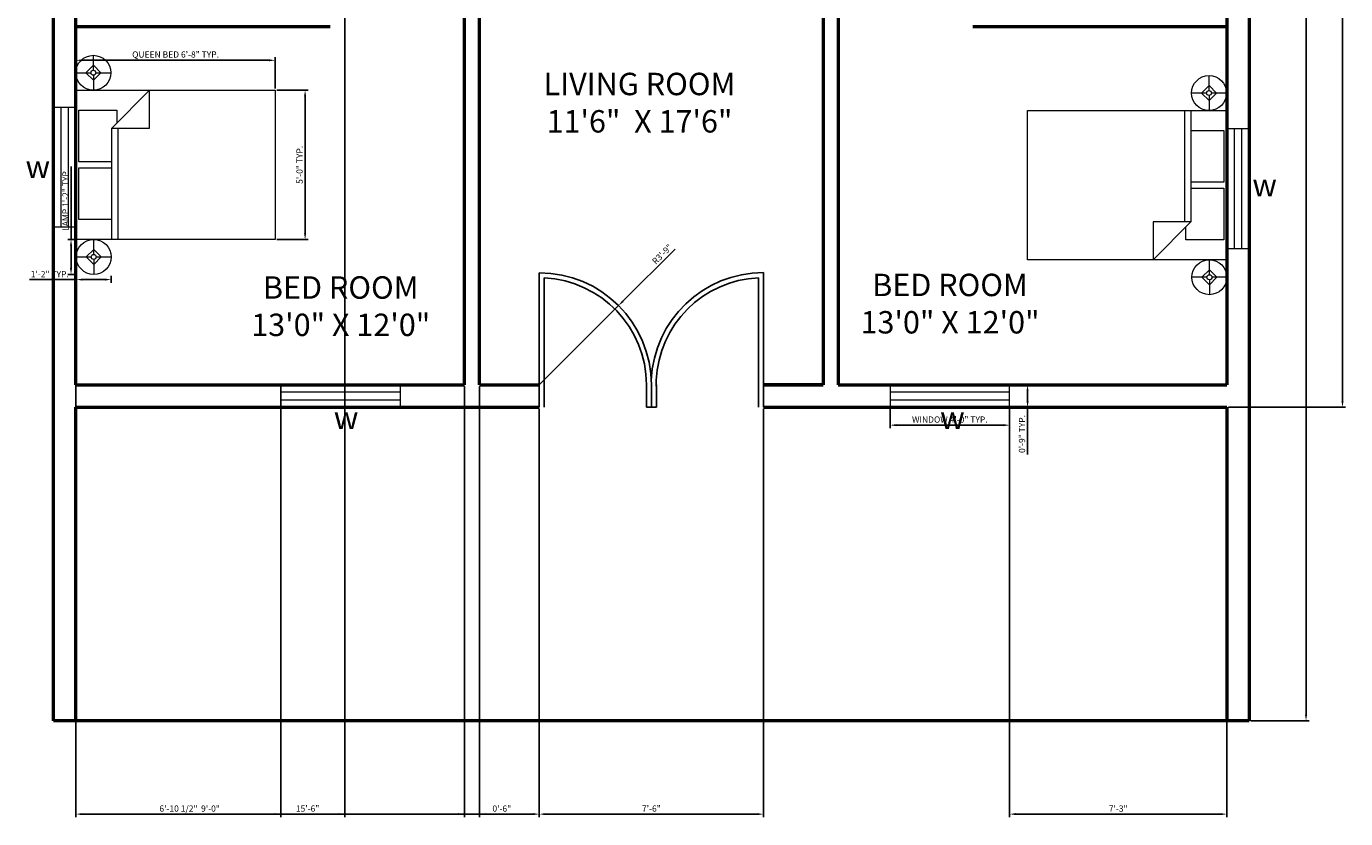
# Model space of a CAD drawing. Units: inches. Extents: x 1776 to 2338, y 1299 to 2099.
# Tile 1 of 4: x 1808 to 2337, y 1299 to 1617. Entities that reach past the tile are written whole.
import ezdxf

# ---------------------------------------------------------------- set-up
doc = ezdxf.new("R2010")
doc.units = ezdxf.units.IN
for name, color, linetype, lineweight in [('A-ANNO-DIMS', 2, 'Continuous', 18), ('A-ANNO-TEXT', 7, 'Continuous', 18), ('A-AREA-IDEN', 7, 'Continuous', 25), ('A-DOOR', 4, 'Continuous', 25), ('A-FURN', 8, 'Continuous', 18), ('A-GLAZ', 4, 'Continuous', 18), ('A-WALL', 7, 'Continuous', 50), ('E-LITE', 9, 'Continuous', 18)]:
    doc.layers.add(name, color=color, linetype=linetype, lineweight=lineweight)
doc.styles.get("Standard").update_dxf_attribs({"font": 'arial.ttf'})
doc.dimstyles.new('ISO-25', dxfattribs={"dimtxt": 2.5, "dimasz": 2.5, "dimexe": 1.25, "dimexo": 0.625, "dimtad": 1, "dimdec": 0, "dimlunit": 3, "dimtxsty": 'Standard', "dimcen": 2.5, "dimadec": 0, "dimazin": 0, "dimtfac": 1, "dimtdec": 0, "dimtmove": 0, "dimatfit": 3, "dimfxl": 1, "dimarcsym": 0})

# ---------------------------------------------------------------- blocks, each defined once
blk = doc.blocks.new('Bed - Queen')
for p, q in [((0, -80.00003), (0, 0)), ((0, 0), (59.99999, 0)), ((59.99999, 0), (59.99999, -80.00003)), ((7.99999, -1.2), (28.79998, -1.2)), ((7.99999, -14.4), (7.99999, -1.2)), ((28.79998, -1.2), (28.79998, -14.4)), ((31.19999, -1.2), (51.99999, -1.2)), ((31.19999, -14.4), (31.19999, -1.2)), ((51.99999, -1.2), (51.99999, -16.4)), ((0, -14.4), (44.8, -14.4)), ((59.99999, -29.6), (44.8, -14.4)), ((44.8, -14.4), (44.8, -29.6)), ((44.8, -16.8), (0, -16.8)), ((51.99999, -16.4), (46.79936, -16.4)), ((44.8, -29.6), (59.99999, -29.6)), ((59.99999, -80.00003), (0, -80.00003))]:
    blk.add_line(p, q)
blk = doc.blocks.new('Lamp - Table')
for p, q in [((0, 7), (0, 1)), ((-1, 0), (-7, 0)), ((0, 3), (-3, 0)), ((-3, 0), (0, -3)), ((3, 0), (0, 3)), ((0, -3), (3, 0)), ((1, 0), (7, 0)), ((0, -1), (0, -7))]:
    blk.add_line(p, q)
for radius in [7, 1]:
    blk.add_circle((0, 0), radius)
blk = doc.blocks.new('*D13')
at = {"layer": 'A-ANNO-DIMS', "color": 0, "lineweight": -2, "transparency": 16777216}
for p, q in [((2299.36, 2058.22), (2322.8, 2058.22)), ((2321.55, 2055.72), (2321.55, 1340.72)), ((2299.36, 1338.22), (2322.8, 1338.22))]:
    blk.add_line(p, q, dxfattribs=at)
at = {"layer": 'A-ANNO-DIMS', "color": 0, "transparency": 16777216}
for points in [[(2321.14, 2055.72), (2321.97, 2055.72), (2321.55, 2058.22)], [(2321.14, 1340.72), (2321.97, 1340.72), (2321.55, 1338.22)]]:
    blk.add_solid(points, dxfattribs=at)
at = {"layer": 'Defpoints', "color": 0, "transparency": 16777216}
for p in [(2298.74, 2058.22), (2298.74, 1338.22), (2321.55, 1338.22)]:
    blk.add_point(p, dxfattribs=at)
at = {"layer": 'A-ANNO-DIMS', "color": 0, "transparency": 16777216, "insert": (2319.65, 1698.22), "char_height": 2.5, "attachment_point": 5, "rotation": 90}
blk.add_mtext("60'", dxfattribs=at)
blk = doc.blocks.new('WIN-48IN')
for p, q in [((48, 9), (0, 9)), ((0, 9), (0, 0)), ((48, 6), (0, 6)), ((48, 0), (48, 9)), ((0, 3), (48, 3)), ((0, 0), (48, 0))]:
    blk.add_line(p, q)
blk = doc.blocks.new('*D18')
at = {"layer": 'A-ANNO-DIMS', "color": 0, "lineweight": -2, "transparency": 16777216}
for p, q in [((2154.56, 1463.59), (2154.56, 1455.77)), ((2202.56, 1463.59), (2202.56, 1455.77)), ((2200.06, 1457.02), (2157.06, 1457.02))]:
    blk.add_line(p, q, dxfattribs=at)
at = {"layer": 'A-ANNO-DIMS', "color": 0, "transparency": 16777216}
for points in [[(2157.06, 1457.44), (2157.06, 1456.6), (2154.56, 1457.02)], [(2200.06, 1457.44), (2200.06, 1456.6), (2202.56, 1457.02)]]:
    blk.add_solid(points, dxfattribs=at)
at = {"layer": 'Defpoints', "color": 0, "transparency": 16777216}
for p in [(2154.56, 1464.22), (2202.56, 1464.22), (2154.56, 1457.02)]:
    blk.add_point(p, dxfattribs=at)
at = {"layer": 'A-ANNO-DIMS', "color": 0, "transparency": 16777216, "insert": (2178.56, 1458.94), "char_height": 2.5, "attachment_point": 5}
blk.add_mtext('WINDOW 4\'-0" TYP.', dxfattribs=at)
blk = doc.blocks.new('*D19')
at = {"layer": 'A-ANNO-DIMS', "color": 0, "lineweight": -2, "transparency": 16777216}
for p, q in [((2203.18, 1473.22), (2211.01, 1473.22)), ((2209.76, 1470.72), (2209.76, 1466.72)), ((2203.18, 1464.22), (2211.01, 1464.22)), ((2209.76, 1464.22), (2209.76, 1445.23))]:
    blk.add_line(p, q, dxfattribs=at)
at = {"layer": 'A-ANNO-DIMS', "color": 0, "transparency": 16777216}
for points in [[(2209.34, 1470.72), (2210.17, 1470.72), (2209.76, 1473.22)], [(2209.34, 1466.72), (2210.17, 1466.72), (2209.76, 1464.22)]]:
    blk.add_solid(points, dxfattribs=at)
at = {"layer": 'Defpoints', "color": 0, "transparency": 16777216}
for p in [(2202.56, 1473.22), (2202.56, 1464.22), (2209.76, 1464.22)]:
    blk.add_point(p, dxfattribs=at)
at = {"layer": 'A-ANNO-DIMS', "color": 0, "transparency": 16777216, "insert": (2207.85, 1453.47), "char_height": 2.5, "attachment_point": 5, "rotation": 90}
blk.add_mtext('0\'-9" TYP.', dxfattribs=at)
blk = doc.blocks.new('*D20')
at = {"layer": 'A-ANNO-DIMS', "color": 0, "lineweight": -2, "transparency": 16777216}
for p, q in [((1825.77, 1531.59), (1825.77, 1560.95)), ((1827.25, 1531.59), (1824.52, 1531.59)), ((1825.77, 1520.09), (1825.77, 1529.09)), ((1827.25, 1517.59), (1824.52, 1517.59))]:
    blk.add_line(p, q, dxfattribs=at)
at = {"layer": 'A-ANNO-DIMS', "color": 0, "transparency": 16777216}
for points in [[(1825.36, 1529.09), (1826.19, 1529.09), (1825.77, 1531.59)], [(1825.36, 1520.09), (1826.19, 1520.09), (1825.77, 1517.59)]]:
    blk.add_solid(points, dxfattribs=at)
at = {"layer": 'Defpoints', "color": 0, "transparency": 16777216}
for p in [(1825.77, 1531.59), (1827.87, 1531.59), (1827.87, 1517.59)]:
    blk.add_point(p, dxfattribs=at)
at = {"layer": 'A-ANNO-DIMS', "color": 0, "transparency": 16777216, "insert": (1823.89, 1547.52), "char_height": 2.5, "attachment_point": 5, "rotation": 90}
blk.add_mtext('LAMP 1\'-2" TYP.', dxfattribs=at)
blk = doc.blocks.new('*D21')
at = {"layer": 'A-ANNO-DIMS', "color": 0, "lineweight": -2, "transparency": 16777216}
for p, q in [((1827.87, 1515.49), (1809.12, 1515.49)), ((1827.87, 1516.97), (1827.87, 1514.24)), ((1839.37, 1515.49), (1830.37, 1515.49)), ((1841.87, 1516.97), (1841.87, 1514.24))]:
    blk.add_line(p, q, dxfattribs=at)
at = {"layer": 'A-ANNO-DIMS', "color": 0, "transparency": 16777216}
for points in [[(1830.37, 1515.91), (1830.37, 1515.08), (1827.87, 1515.49)], [(1839.37, 1515.91), (1839.37, 1515.08), (1841.87, 1515.49)]]:
    blk.add_solid(points, dxfattribs=at)
at = {"layer": 'Defpoints', "color": 0, "transparency": 16777216}
for p in [(1827.87, 1517.59), (1827.87, 1515.49), (1841.87, 1517.59)]:
    blk.add_point(p, dxfattribs=at)
at = {"layer": 'A-ANNO-DIMS', "color": 0, "transparency": 16777216, "insert": (1817.25, 1517.37), "char_height": 2.5, "attachment_point": 5}
blk.add_mtext('1\'-2" TYP.', dxfattribs=at)
blk = doc.blocks.new('*D24')
at = {"layer": 'A-ANNO-DIMS', "color": 0, "lineweight": -2, "transparency": 16777216}
for p, q in [((1827.74, 1592.22), (1827.74, 1604.84)), ((1907.74, 1592.22), (1907.74, 1604.84)), ((1905.24, 1603.59), (1830.24, 1603.59))]:
    blk.add_line(p, q, dxfattribs=at)
at = {"layer": 'A-ANNO-DIMS', "color": 0, "transparency": 16777216}
for points in [[(1830.24, 1604.01), (1830.24, 1603.18), (1827.74, 1603.59)], [(1905.24, 1604.01), (1905.24, 1603.18), (1907.74, 1603.59)]]:
    blk.add_solid(points, dxfattribs=at)
at = {"layer": 'Defpoints', "color": 0, "transparency": 16777216}
for p in [(1827.74, 1603.59), (1827.74, 1591.59), (1907.74, 1591.59)]:
    blk.add_point(p, dxfattribs=at)
at = {"layer": 'A-ANNO-DIMS', "color": 0, "transparency": 16777216, "insert": (1867.74, 1605.59), "char_height": 2.5, "attachment_point": 5}
blk.add_mtext('QUEEN BED 6\'-8" TYP.', dxfattribs=at)
blk = doc.blocks.new('*D25')
at = {"layer": 'A-ANNO-DIMS', "color": 0, "lineweight": -2, "transparency": 16777216}
for p, q in [((1908.36, 1591.59), (1920.99, 1591.59)), ((1919.74, 1534.09), (1919.74, 1589.09)), ((1908.36, 1531.59), (1920.99, 1531.59))]:
    blk.add_line(p, q, dxfattribs=at)
at = {"layer": 'A-ANNO-DIMS', "color": 0, "transparency": 16777216}
for points in [[(1919.32, 1589.09), (1920.16, 1589.09), (1919.74, 1591.59)], [(1919.32, 1534.09), (1920.16, 1534.09), (1919.74, 1531.59)]]:
    blk.add_solid(points, dxfattribs=at)
at = {"layer": 'Defpoints', "color": 0, "transparency": 16777216}
for p in [(1907.74, 1591.59), (1919.74, 1591.59), (1907.74, 1531.59)]:
    blk.add_point(p, dxfattribs=at)
at = {"layer": 'A-ANNO-DIMS', "color": 0, "transparency": 16777216, "insert": (1917.84, 1561.59), "char_height": 2.5, "attachment_point": 5, "rotation": 90}
blk.add_mtext('5\'-0" TYP.', dxfattribs=at)
blk = doc.blocks.new('*D42')
at = {"layer": 'A-ANNO-DIMS', "color": 0, "lineweight": -2, "transparency": 16777216}
for p, q in [((2299.36, 2058.22), (2337.44, 2058.22)), ((2336.19, 1466.72), (2336.19, 2055.72)), ((2290.36, 1464.22), (2337.44, 1464.22))]:
    blk.add_line(p, q, dxfattribs=at)
at = {"layer": 'A-ANNO-DIMS', "color": 0, "transparency": 16777216}
for points in [[(2335.77, 2055.72), (2336.61, 2055.72), (2336.19, 2058.22)], [(2335.77, 1466.72), (2336.61, 1466.72), (2336.19, 1464.22)]]:
    blk.add_solid(points, dxfattribs=at)
at = {"layer": 'Defpoints', "color": 0, "transparency": 16777216}
for p in [(2298.74, 2058.22), (2336.19, 2058.22), (2289.74, 1464.22)]:
    blk.add_point(p, dxfattribs=at)
at = {"layer": 'A-ANNO-DIMS', "color": 0, "transparency": 16777216, "insert": (2334.29, 1761.22), "char_height": 2.5, "attachment_point": 5, "rotation": 90}
blk.add_mtext('49\'-6"', dxfattribs=at)
blk = doc.blocks.new('*D43')
at = {"layer": 'A-ANNO-DIMS', "color": 0, "lineweight": -2, "transparency": 16777216}
for p, q in [((2013.74, 1463.59), (2013.74, 1299.52)), ((2103.74, 1463.59), (2103.74, 1299.52)), ((2016.24, 1300.77), (2101.24, 1300.77))]:
    blk.add_line(p, q, dxfattribs=at)
at = {"layer": 'A-ANNO-DIMS', "color": 0, "transparency": 16777216}
for points in [[(2016.24, 1301.19), (2016.24, 1300.35), (2013.74, 1300.77)], [(2101.24, 1301.19), (2101.24, 1300.35), (2103.74, 1300.77)]]:
    blk.add_solid(points, dxfattribs=at)
at = {"layer": 'Defpoints', "color": 0, "transparency": 16777216}
for p in [(2013.74, 1464.22), (2103.74, 1464.22), (2103.74, 1300.77)]:
    blk.add_point(p, dxfattribs=at)
at = {"layer": 'A-ANNO-DIMS', "color": 0, "transparency": 16777216, "insert": (2058.74, 1302.67), "char_height": 2.5, "attachment_point": 5}
blk.add_mtext('7\'-6"', dxfattribs=at)
blk = doc.blocks.new('*D44')
at = {"layer": 'A-ANNO-DIMS', "color": 0, "lineweight": -2, "transparency": 16777216}
for p, q in [((1827.74, 1463.59), (1827.74, 1299.52)), ((2013.74, 1463.59), (2013.74, 1299.52)), ((1830.24, 1300.77), (2011.24, 1300.77))]:
    blk.add_line(p, q, dxfattribs=at)
at = {"layer": 'A-ANNO-DIMS', "color": 0, "transparency": 16777216}
for points in [[(1830.24, 1301.19), (1830.24, 1300.35), (1827.74, 1300.77)], [(2011.24, 1301.19), (2011.24, 1300.35), (2013.74, 1300.77)]]:
    blk.add_solid(points, dxfattribs=at)
at = {"layer": 'Defpoints', "color": 0, "transparency": 16777216}
for p in [(1827.74, 1464.22), (2013.74, 1464.22), (2013.74, 1300.77)]:
    blk.add_point(p, dxfattribs=at)
at = {"layer": 'A-ANNO-DIMS', "color": 0, "transparency": 16777216, "insert": (1920.74, 1302.67), "char_height": 2.5, "attachment_point": 5}
blk.add_mtext('15\'-6"', dxfattribs=at)
blk = doc.blocks.new('*D47')
at = {"layer": 'A-ANNO-DIMS', "color": 0, "lineweight": -2, "transparency": 16777216}
for p, q in [((1827.74, 1688.59), (1827.74, 1299.52)), ((1935.74, 1688.59), (1935.74, 1299.52)), ((1830.24, 1300.77), (1933.24, 1300.77))]:
    blk.add_line(p, q, dxfattribs=at)
at = {"layer": 'A-ANNO-DIMS', "color": 0, "transparency": 16777216}
for points in [[(1830.24, 1301.19), (1830.24, 1300.35), (1827.74, 1300.77)], [(1933.24, 1301.19), (1933.24, 1300.35), (1935.74, 1300.77)]]:
    blk.add_solid(points, dxfattribs=at)
at = {"layer": 'Defpoints', "color": 0, "transparency": 16777216}
for p in [(1827.74, 1689.22), (1935.74, 1689.22), (1935.74, 1300.77)]:
    blk.add_point(p, dxfattribs=at)
at = {"layer": 'A-ANNO-DIMS', "color": 0, "transparency": 16777216, "insert": (1881.74, 1302.67), "char_height": 2.5, "attachment_point": 5}
blk.add_mtext('9\'-0"', dxfattribs=at)
blk = doc.blocks.new('*D50')
at = {"layer": 'A-ANNO-DIMS', "color": 0, "lineweight": -2, "transparency": 16777216}
for p, q in [((1983.74, 1472.59), (1983.74, 1299.52)), ((1989.74, 1472.59), (1989.74, 1299.52)), ((1981.24, 1300.77), (1978.74, 1300.77)), ((1983.74, 1300.77), (1989.74, 1300.77)), ((1992.24, 1300.77), (2002.63, 1300.77))]:
    blk.add_line(p, q, dxfattribs=at)
at = {"layer": 'A-ANNO-DIMS', "color": 0, "transparency": 16777216}
for points in [[(1981.24, 1301.19), (1981.24, 1300.35), (1983.74, 1300.77)], [(1992.24, 1301.19), (1992.24, 1300.35), (1989.74, 1300.77)]]:
    blk.add_solid(points, dxfattribs=at)
at = {"layer": 'Defpoints', "color": 0, "transparency": 16777216}
for p in [(1983.74, 1473.22), (1989.74, 1473.22), (1989.74, 1300.77)]:
    blk.add_point(p, dxfattribs=at)
at = {"layer": 'A-ANNO-DIMS', "color": 0, "transparency": 16777216, "insert": (1998.69, 1302.67), "char_height": 2.5, "attachment_point": 5}
blk.add_mtext('0\'-6"', dxfattribs=at)
blk = doc.blocks.new('*D55')
at = {"layer": 'A-ANNO-DIMS', "color": 0, "lineweight": -2, "transparency": 16777216}
for p, q in [((1827.74, 1472.59), (1827.74, 1299.52)), ((1910.05, 1472.59), (1910.05, 1299.52)), ((1830.24, 1300.77), (1907.55, 1300.77))]:
    blk.add_line(p, q, dxfattribs=at)
at = {"layer": 'A-ANNO-DIMS', "color": 0, "transparency": 16777216}
for points in [[(1830.24, 1301.19), (1830.24, 1300.35), (1827.74, 1300.77)], [(1907.55, 1301.19), (1907.55, 1300.35), (1910.05, 1300.77)]]:
    blk.add_solid(points, dxfattribs=at)
at = {"layer": 'Defpoints', "color": 0, "transparency": 16777216}
for p in [(1827.74, 1473.22), (1910.05, 1473.22), (1910.05, 1300.77)]:
    blk.add_point(p, dxfattribs=at)
at = {"layer": 'A-ANNO-DIMS', "color": 0, "transparency": 16777216, "insert": (1868.89, 1302.69), "char_height": 2.5, "attachment_point": 5}
blk.add_mtext('6\'-10 1/2"', dxfattribs=at)
blk = doc.blocks.new('*D56')
at = {"layer": 'A-ANNO-DIMS', "color": 0, "lineweight": -2, "transparency": 16777216}
for p, q in [((2202.56, 1463.59), (2202.56, 1299.52)), ((2289.74, 1463.59), (2289.74, 1299.52)), ((2205.06, 1300.77), (2287.24, 1300.77))]:
    blk.add_line(p, q, dxfattribs=at)
at = {"layer": 'A-ANNO-DIMS', "color": 0, "transparency": 16777216}
for points in [[(2205.06, 1301.19), (2205.06, 1300.35), (2202.56, 1300.77)], [(2287.24, 1301.19), (2287.24, 1300.35), (2289.74, 1300.77)]]:
    blk.add_solid(points, dxfattribs=at)
at = {"layer": 'Defpoints', "color": 0, "transparency": 16777216}
for p in [(2202.56, 1464.22), (2289.74, 1464.22), (2289.74, 1300.77)]:
    blk.add_point(p, dxfattribs=at)
at = {"layer": 'A-ANNO-DIMS', "color": 0, "transparency": 16777216, "insert": (2246.15, 1302.67), "char_height": 2.5, "attachment_point": 5}
blk.add_mtext('7\'-3"', dxfattribs=at)
blk = doc.blocks.new('*D58')
at = {"layer": 'A-ANNO-DIMS', "color": 0, "lineweight": -2, "transparency": 16777216}
for p, q in [((2068.29, 1527.77), (2047.33, 1506.81)), ((2013.74, 1473.22), (2045.56, 1505.04))]:
    blk.add_line(p, q, dxfattribs=at)
at = {"layer": 'A-ANNO-DIMS', "color": 0, "transparency": 16777216}
blk.add_solid([(2047.03, 1507.1), (2047.62, 1506.51), (2045.56, 1505.04)], dxfattribs=at)
at = {"layer": 'Defpoints', "color": 0, "transparency": 16777216}
for p in [(2045.56, 1505.04), (2013.74, 1473.22)]:
    blk.add_point(p, dxfattribs=at)
at = {"layer": 'A-ANNO-DIMS', "color": 0, "transparency": 16777216, "insert": (2063.31, 1525.48), "char_height": 2.5, "attachment_point": 5, "rotation": 45.0001}
blk.add_mtext('R3\'-9"', dxfattribs=at)

msp = doc.modelspace()

# ---------------------------------------------------------------- linework, layer by layer
at = {"layer": 'A-DOOR'}
for p, q in [((2013.74, 1473.22), (2013.74, 1518.22)), ((2015.74, 1518.17), (2015.74, 1518.22)), ((2015.74, 1473.22), (2015.74, 1516.17)), ((2101.74, 1473.22), (2101.74, 1516.25)), ((2103.74, 1473.22), (2103.74, 1518.3)), ((2013.74, 1473.22), (2013.74, 1464.22)), ((2015.74, 1473.22), (2015.74, 1464.22)), ((2056.74, 1473.22), (2056.74, 1464.22)), ((2058.74, 1473.22), (2058.74, 1464.22)), ((2058.74, 1473.22), (2058.74, 1464.22)), ((2060.7, 1475.05), (2060.74, 1469.97)), ((2060.74, 1473.22), (2060.74, 1464.22)), ((2101.74, 1473.22), (2101.74, 1464.22)), ((2103.74, 1473.22), (2103.74, 1464.22)), ((2056.74, 1464.22), (2058.74, 1464.22)), ((2058.74, 1464.22), (2060.74, 1464.22))]:
    msp.add_line(p, q, dxfattribs=at)
for centre, radius, start, end in [((2013.74, 1473.22), 45, 0, 90), ((2013.74, 1473.22), 43, 0, 87.3341), ((2103.74, 1473.22), 45.08, 90, 177.5604), ((2103.74, 1473.22), 43.08, 92.6608, 177.5604)]:
    msp.add_arc(centre, radius, start, end, dxfattribs=at)
at = {"layer": 'A-WALL'}
for p, q in [((1818.74, 1338.22), (1818.74, 2058.22)), ((2298.74, 2058.22), (2298.74, 1338.22)), ((2289.74, 1899.22), (2289.74, 1473.22)), ((1827.74, 1473.22), (1827.74, 1833.22)), ((1983.74, 1473.22), (1983.74, 1683.22)), ((1989.74, 1473.22), (1989.74, 1683.22)), ((2127.74, 1683.22), (2127.74, 1473.22)), ((2133.74, 1683.22), (2133.74, 1473.22)), ((1827.74, 1617.22), (1929.74, 1617.22)), ((2187.74, 1617.22), (2289.74, 1617.22)), ((1827.74, 1473.22), (1929.74, 1473.22)), ((1929.74, 1473.22), (1983.74, 1473.22)), ((1989.74, 1473.22), (2013.74, 1473.22)), ((1989.74, 1473.22), (2013.74, 1473.22)), ((2127.74, 1473.22), (2103.74, 1473.22)), ((2103.74, 1473.22), (2127.74, 1473.22)), ((2127.74, 1473.22), (2115.74, 1473.22)), ((2127.74, 1473.22), (2127.74, 1473.22)), ((2133.74, 1473.22), (2187.74, 1473.22)), ((2187.74, 1473.22), (2289.74, 1473.22)), ((1827.74, 1338.22), (1827.74, 1464.22)), ((1827.74, 1464.22), (1929.74, 1464.22)), ((1929.74, 1464.22), (2013.74, 1464.22)), ((2103.74, 1464.22), (2187.74, 1464.22)), ((2187.74, 1464.22), (2289.74, 1464.22)), ((2289.74, 1464.22), (2289.74, 1338.22)), ((2298.74, 1338.22), (1818.74, 1338.22))]:
    msp.add_line(p, q, dxfattribs=at)

# ---------------------------------------------------------------- block references
at = {"layer": 'A-FURN'}
for p, rotation in [((1827.74, 1531.59), 89.99999999999999), ((2289.74, 1583.44), 270)]:
    msp.add_blockref('Bed - Queen', p, dxfattribs=dict(at, rotation=rotation))
at = {"layer": 'A-GLAZ'}
for p, rotation in [((1818.74, 1584.63), 269.9999999999979), ((2289.74, 1576.05), 269.999999999997), ((1958.05, 1473.22), 180), ((2202.56, 1473.22), 180)]:
    msp.add_blockref('WIN-48IN', p, dxfattribs=dict(at, rotation=rotation))
at = {"layer": 'E-LITE'}
for p, rotation in [((1834.73, 1598.59), 89.99999999999999), ((2282.6, 1590.44), 270), ((1834.87, 1524.59), 89.99999999999999), ((2282.75, 1516.44), 270)]:
    msp.add_blockref('Lamp - Table', p, dxfattribs=dict(at, rotation=rotation))

# ---------------------------------------------------------------- texts
at = {"layer": 'A-ANNO-TEXT', "char_height": 9, "attachment_point": 1}
for insert in [(1787.33, 1565.36), (2279.82, 1558), (1911.09, 1464.45), (2154.48, 1464.45)]:
    msp.add_mtext_dynamic_manual_height_columns('\\pxqc;w', width=50.2204, gutter_width=12.5, heights=[0], dxfattribs=dict(at, insert=insert))
at = {"layer": 'A-AREA-IDEN', "char_height": 9, "attachment_point": 1}
for s, insert in [('\\pxqc;LIVING ROOM\\P11\'6"  X 17\'6"', (2001.26, 1598.57)), ('\\pxqc;BED ROOM \\P13\'0" X 12\'0"', (1881.33, 1516.82)), ('\\pxqc;BED ROOM \\P13\'0" X 12\'0"', (2125.92, 1517.85))]:
    msp.add_mtext_dynamic_manual_height_columns(s, width=105.4264, gutter_width=12.5, heights=[0], dxfattribs=dict(at, insert=insert))

# ---------------------------------------------------------------- dimensions: what is measured, and where the dimension line sits
at = {"layer": 'A-ANNO-DIMS'}
for base, p1, p2, override, picture, middle in [((2336.19, 2058.22), (2289.74, 1464.22), (2298.74, 2058.22), {"dimdec": 1, "dimlfac": 1, "dimrnd": 0, "dimzin": 1, "dimdsep": 46, "dimlunit": 4, "dimfrac": 2}, '*D42', (2334.29, 1761.22)), ((2321.55, 1338.22), (2298.74, 2058.22), (2298.74, 1338.22), {"dimclrd": 0, "dimclre": 0, "dimclrt": 0}, '*D13', (2319.65, 1698.22))]:
    dim = msp.add_linear_dim(base=base, p1=p1, p2=p2, angle=90, dimstyle='ISO-25', override=override, dxfattribs=at)
    dim.commit()
    dim.dimension.update_dxf_attribs({"geometry": picture, "text_midpoint": middle})
for base, p1, p2, picture, middle in [((1935.74, 1300.77), (1827.74, 1689.22), (1935.74, 1689.22), '*D47', (1881.74, 1302.67)), ((1910.05, 1300.77), (1827.74, 1473.22), (1910.05, 1473.22), '*D55', (1868.89, 1302.69)), ((1989.74, 1300.77), (1983.74, 1473.22), (1989.74, 1473.22), '*D50', (1998.69, 1302.67)), ((2013.74, 1300.77), (1827.74, 1464.22), (2013.74, 1464.22), '*D44', (1920.74, 1302.67)), ((2103.74, 1300.77), (2013.74, 1464.22), (2103.74, 1464.22), '*D43', (2058.74, 1302.67)), ((2289.74, 1300.77), (2202.56, 1464.22), (2289.74, 1464.22), '*D56', (2246.15, 1302.67))]:
    dim = msp.add_linear_dim(base=base, p1=p1, p2=p2, dimstyle='ISO-25', override={"dimdec": 1, "dimlfac": 1, "dimrnd": 0, "dimzin": 1, "dimdsep": 46, "dimlunit": 4, "dimfrac": 2}, dxfattribs=at)
    dim.commit()
    dim.dimension.update_dxf_attribs({"geometry": picture, "text_midpoint": middle})
for base, p1, p2, angle, text, picture, middle in [((1827.74, 1603.59), (1907.74, 1591.59), (1827.74, 1591.59), 180, 'QUEEN BED <> TYP.', '*D24', (1867.74, 1605.59)), ((1919.74, 1591.59), (1907.74, 1531.59), (1907.74, 1591.59), 90, '<> TYP.', '*D25', (1917.84, 1561.59)), ((1825.77, 1531.59), (1827.87, 1517.59), (1827.87, 1531.59), 90, 'LAMP <> TYP.', '*D20', (1823.89, 1547.52)), ((1827.87, 1515.49), (1841.87, 1517.59), (1827.87, 1517.59), 180, '<> TYP.', '*D21', (1817.25, 1517.37)), ((2209.76, 1464.22), (2202.56, 1473.22), (2202.56, 1464.22), 270, '<> TYP.', '*D19', (2207.85, 1453.47)), ((2154.56, 1457.02), (2202.56, 1464.22), (2154.56, 1464.22), 180, 'WINDOW <> TYP.', '*D18', (2178.56, 1458.94))]:
    dim = msp.add_linear_dim(base=base, p1=p1, p2=p2, angle=angle, text=text, dimstyle='ISO-25', override={"dimdec": 1, "dimlfac": 1, "dimrnd": 0, "dimzin": 1, "dimdsep": 46, "dimlunit": 4, "dimfrac": 2}, dxfattribs=at)
    dim.commit()
    dim.dimension.update_dxf_attribs({"geometry": picture, "text_midpoint": middle})
dim = msp.add_radius_dim(center=(2013.74, 1473.22), mpoint=(2045.56, 1505.04), dimstyle='ISO-25', override={"dimdec": 1, "dimlfac": 1, "dimrnd": 0, "dimzin": 1, "dimdsep": 46, "dimlunit": 4, "dimfrac": 2}, dxfattribs=at)
dim.commit()
dim.dimension.update_dxf_attribs({"geometry": '*D58', "text_midpoint": (2064.65, 1524.13), "dimtype": 164})

doc.saveas('drawing.dxf')
